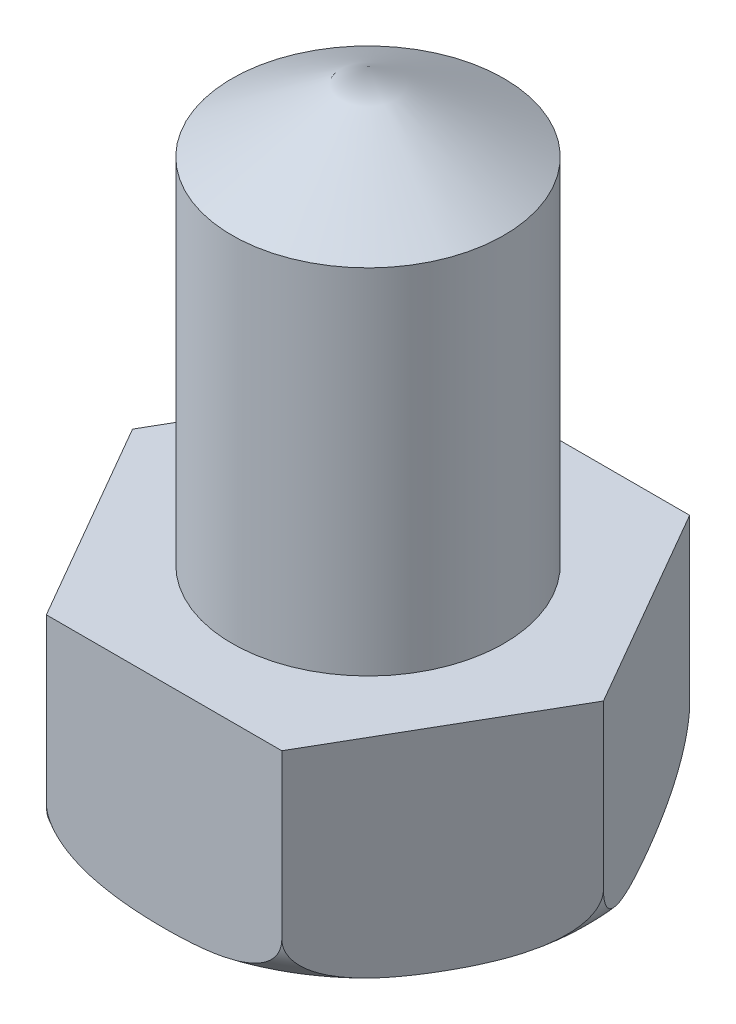
from build123d import *

# Parameters (mm, degrees)
HEX_HEAD_15AF_DEPTH = 8


with BuildPart() as part:
    # Hex Head Profile → Hex Head 15AF (new body)
    with BuildSketch(Plane(origin=(0, 0, 0), x_dir=(1, 0, 0), z_dir=(0, 1, 0))):
        Polygon((8.660254038, 0), (4.330127019, 7.5), (-4.330127019, 7.5), (-8.660254038, 0), (-4.330127019, -7.5), (4.330127019, -7.5), align=None)
    extrude(amount=HEX_HEAD_15AF_DEPTH)

    # Shank Profile → Shank with Cone Point (revolve)
    with BuildSketch(Plane.XY, mode=Mode.PRIVATE) as shank_with_cone_point_sk:
        Polygon((0, 8), (0, 23.886751346), (5, 21), (5, 8), align=None)
    revolve(shank_with_cone_point_sk.sketch.rotate(Axis((0, 23.886751346, 0), (0, 1, 0)), 90), axis=Axis((0, 23.886751346, 0), (0, 1, 0)))

    # Head Chamfer Profile → Head Chamfer Cut (revolve, cut)
    with BuildSketch(Plane.XY, mode=Mode.PRIVATE) as head_chamfer_cut_sk:
        with BuildLine():
            Line((8.660254038, 0), (6.660254038, 0))
            ThreePointArc((6.660254038, 0), (8.0744676, 0.585786438), (8.660254038, 2))
            Line((8.660254038, 2), (8.660254038, 0))
        make_face()
    revolve(head_chamfer_cut_sk.sketch.rotate(Axis((0, 0, 0), (0, 1, 0)), 90), axis=Axis((0, 0, 0), (0, 1, 0)), mode=Mode.SUBTRACT)


solid = part.part
